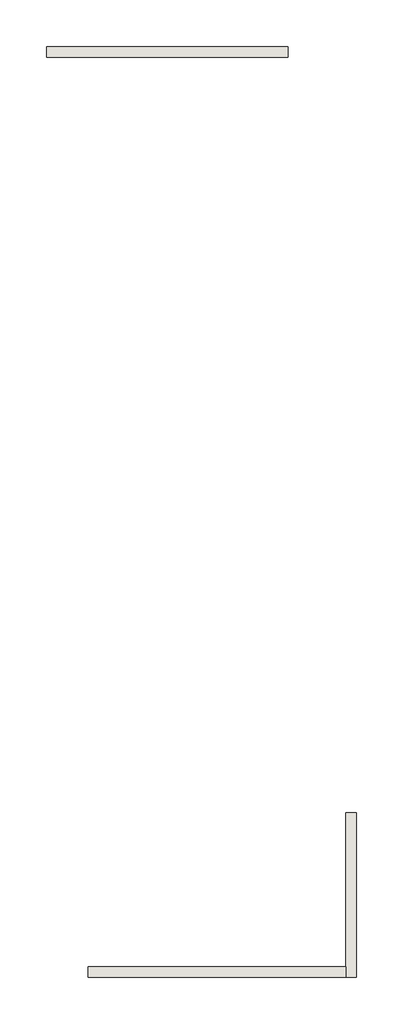
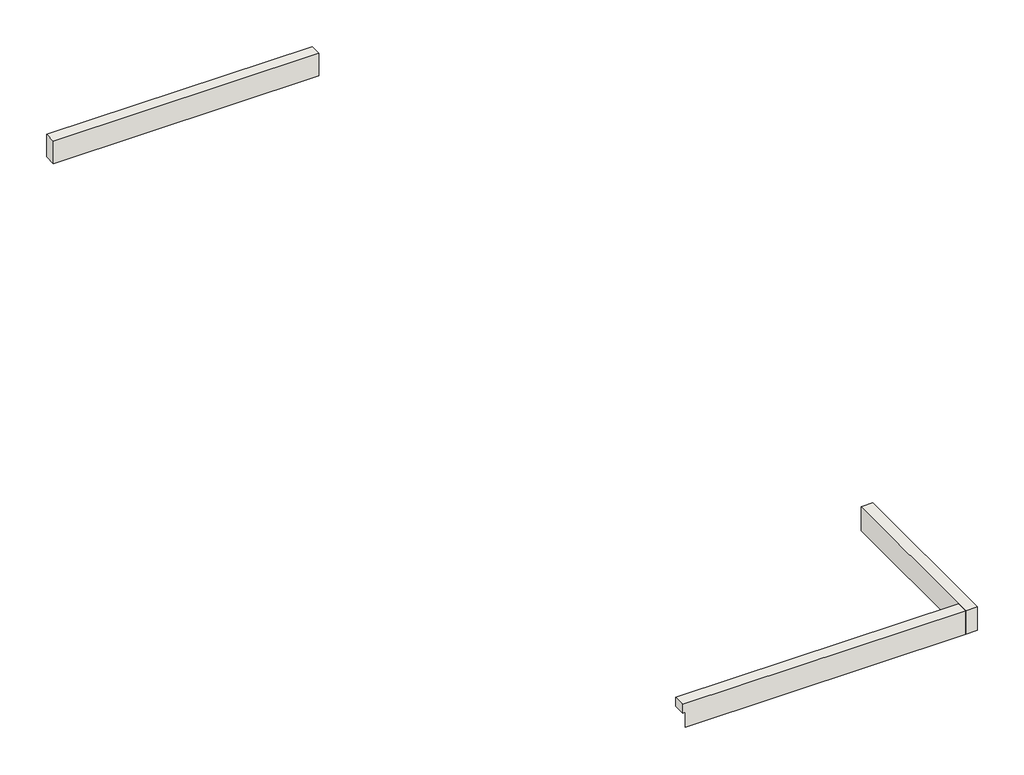
# One storey: 3 walls.
"""IFC4 building model written with IfcOpenShell, lengths in millimetres."""

from ifc_helpers import new_model, si_unit, frame, origin, place, context, project, spatial, polyline, outline, extrude, faceted_brep, element, save

model = new_model("IFC4")

# Units and contexts
model_context = context("Model", 3, world=origin())
ifc_project = project(units=[si_unit("LENGTHUNIT", "METRE", prefix="MILLI")], contexts=[model_context])

# Site, building, storey
site = spatial("IfcSite", under=ifc_project)
building = spatial("IfcBuilding", under=site)
storey = spatial("IfcBuildingStorey", under=building, Elevation=3900.0)

# Walls
placement = place(None, origin())
element("IfcWall", 1, ObjectType="01-225 wall", at=placement, inside=storey, context=model_context, shape_type="Brep", body=[
    faceted_brep([(-2660.4564803, -10622.5265, 3900.0), (-2660.4564803, -13822.5265, 3900.0), (-2660.4564803, -14047.5265, 3900.0), (-2660.4564803, -14047.5265, 4375.0), (-2660.4564803, -13822.5265, 4375.0), (-2660.4564803, -10622.5265, 4375.0), (-2435.4564803, -10622.5265, 3900.0), (-2435.4564803, -10622.5265, 4375.0), (-2435.4564803, -14047.5265, 4375.0), (-2435.4564803, -14047.5265, 3900.0)], [[[0, 1, 2, 3, 4, 5]], [[6, 7, 8, 9]], [[2, 1, 0, 6, 9]], [[5, 4, 3, 8, 7]], [[0, 5, 7, 6]], [[3, 2, 9, 8]]]),
])
element("IfcWall", 2, ObjectType="01-225 wall", at=placement, inside=storey, context=model_context, shape_type="Brep", body=[
    faceted_brep([(-2660.4564803, -13822.5265, 3900.0), (-7742.2584287, -13822.5265, 3900.0), (-7742.2584287, -13822.5265, 4200.0), (-8013.8574545, -13822.5265, 4200.0), (-8013.8574545, -13822.5265, 4350.0), (-8013.8574545, -13822.5265, 4375.0), (-2660.4564803, -13822.5265, 4375.0), (-2660.4564803, -14047.5265, 3900.0), (-2660.4564803, -14047.5265, 4375.0), (-8013.8574545, -14047.5265, 4375.0), (-8013.8574545, -14047.5265, 4350.0), (-8013.8574545, -14047.5265, 4200.0), (-7967.2584287, -14047.5265, 4200.0), (-7967.2584287, -14047.5265, 3900.0)], [[[0, 1, 2, 3, 4, 5, 6]], [[7, 8, 9, 10, 11, 12, 13]], [[1, 0, 7, 13]], [[6, 5, 9, 8]], [[0, 6, 8, 7]], [[5, 4, 3, 11, 10, 9]], [[11, 3, 2, 12]], [[2, 1, 13, 12]]]),
])
element("IfcWall", 3, ObjectType="01-225 wall", at=placement, inside=storey, context=model_context, shape_type="SweptSolid", body=[
    extrude(outline(polyline([(-3860.4564803, 5077.4735), (-8885.4564803, 5077.4735), (-8885.4564803, 5302.4735), (-3860.4564803, 5302.4735), (-3860.4564803, 5077.4735)])), frame((0.0, 0.0, 3900.0), z_axis=(0.0, 0.0, 1.0), x_axis=(1.0, 0.0, 0.0)), (0.0, 0.0, 1.0), 450.0),
])

save(model, "model.ifc")

# Revit data of these elements
# Type "01-225 wall"
#   Description = "Generic Wall (Material By Category), 200mm thick"
#   Assembly Code = "B2010"
#   Type Mark = "G06"
#   Layers, outside or top first: 225 mm "01-225 wall paint" (function 1)
# Elements 1, 2 (IfcWall, "01-225 wall")
#   Top Offset = 25 mm
#   Base Offset = 0 mm
#   wall height = 475 mm
#   Phase Created = New Construction
#   Top Constraint = 05-ROOF
#   Materials on its faces: "01-225 wall paint"
# Element 3 (IfcWall, "01-225 wall")
#   Top Offset = 0 mm
#   Base Offset = 0 mm
#   wall height = 450 mm
#   Phase Created = New Construction
#   Top Constraint = 05-ROOF
#   Materials on its faces: "01-225 wall paint"
# Materials
#   "01-225 wall paint": class "Generic", colour RGB 242 242 255, transparency 0, Cost = 0
